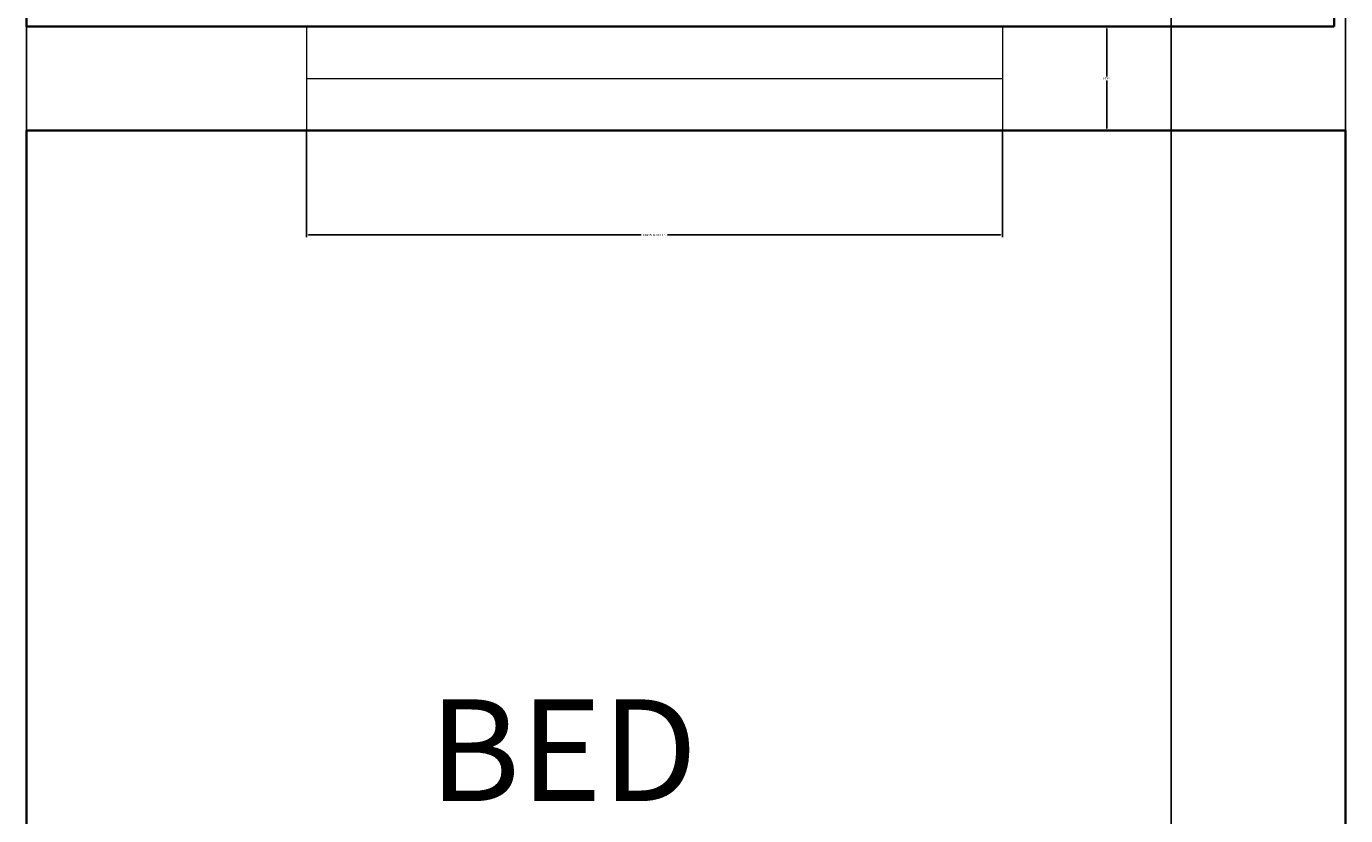
# Model space of a CAD drawing. Units: feet. Extents: x 100807 to 101423, y 154875 to 156331.
# Tile 5 of 8: x 101058 to 101172, y 156097 to 156166. Entities that reach past the tile are written whole.
import ezdxf

# ---------------------------------------------------------------- set-up
doc = ezdxf.new("R2010")
doc.units = ezdxf.units.FT
for name, color, linetype, lineweight in [('A-ANNO-DIMS', 2, 'Continuous', 18), ('A-AREA-IDEN', 7, 'Continuous', 25), ('A-GLAZ', 4, 'Continuous', 18), ('A-WALL', 7, 'Continuous', 35)]:
    doc.layers.add(name, color=color, linetype=linetype, lineweight=lineweight)
doc.styles.get("Standard").update_dxf_attribs({"font": 'arial.ttf'})
doc.dimstyles.get("Standard").update_dxf_attribs({"dimtxt": 0.18, "dimasz": 0.18, "dimexe": 0.18, "dimexo": 0.0625, "dimgap": 0.09, "dimtad": 0, "dimtih": 1, "dimtoh": 1, "dimdec": 4, "dimzin": 0, "dimdsep": 46, "dimtxsty": 'Standard', "dimcen": 0.09, "dimadec": 0, "dimazin": 0, "dimtfac": 1, "dimtdec": 4, "dimtofl": 0, "dimtmove": 0, "dimatfit": 3, "dimfxl": 1, "dimtolj": 1, "dimtzin": 0, "dimarcsym": 0})

# ---------------------------------------------------------------- blocks, each defined once
blk = doc.blocks.new('WIN-BED-END')
for p, q in [((0, 9), (0, 0)), ((60.14, 9), (60.14, 0)), ((0, 4.5), (60.14, 4.5))]:
    blk.add_line(p, q)
blk = doc.blocks.new('*D28')
at = {"layer": 'A-ANNO-DIMS', "color": 0, "lineweight": -2, "transparency": 16777216}
for p, q in [((101082.36, 156156.52), (101082.36, 156147.38)), ((101142.5, 156156.52), (101142.5, 156147.38)), ((101082.54, 156147.56), (101111.29, 156147.56)), ((101142.32, 156147.56), (101113.57, 156147.56))]:
    blk.add_line(p, q, dxfattribs=at)
at = {"layer": 'A-ANNO-DIMS', "color": 0, "transparency": 16777216}
for points in [[(101082.54, 156147.59), (101082.54, 156147.53), (101082.36, 156147.56)], [(101142.32, 156147.59), (101142.32, 156147.53), (101142.5, 156147.56)]]:
    blk.add_solid(points, dxfattribs=at)
at = {"layer": 'Defpoints', "color": 0, "transparency": 16777216}
for p in [(101082.36, 156156.58), (101142.5, 156156.58), (101142.5, 156147.56)]:
    blk.add_point(p, dxfattribs=at)
at = {"layer": 'A-ANNO-DIMS', "color": 0, "transparency": 16777216, "insert": (101112.43, 156147.56), "char_height": 0.18, "attachment_point": 5}
blk.add_mtext('\\A1;END WIN. 60 TYP.', dxfattribs=at)
blk = doc.blocks.new('*D29')
at = {"layer": 'A-ANNO-DIMS', "color": 0, "lineweight": -2, "transparency": 16777216}
for p, q in [((101142.56, 156165.58), (101151.7, 156165.58)), ((101151.52, 156165.4), (101151.52, 156161.26)), ((101151.52, 156156.76), (101151.52, 156160.9)), ((101142.56, 156156.58), (101151.7, 156156.58))]:
    blk.add_line(p, q, dxfattribs=at)
at = {"layer": 'A-ANNO-DIMS', "color": 0, "transparency": 16777216}
for points in [[(101151.49, 156165.4), (101151.55, 156165.4), (101151.52, 156165.58)], [(101151.49, 156156.76), (101151.55, 156156.76), (101151.52, 156156.58)]]:
    blk.add_solid(points, dxfattribs=at)
at = {"layer": 'Defpoints', "color": 0, "transparency": 16777216}
for p in [(101142.5, 156165.58), (101151.52, 156165.58), (101142.5, 156156.58)]:
    blk.add_point(p, dxfattribs=at)
at = {"layer": 'A-ANNO-DIMS', "color": 0, "transparency": 16777216, "insert": (101151.52, 156161.08), "char_height": 0.18, "attachment_point": 5}
blk.add_mtext('\\A1;9 TYP.', dxfattribs=at)
blk = doc.blocks.new('*D36')
at = {"layer": 'A-ANNO-DIMS', "color": 0, "lineweight": -2, "transparency": 16777216}
for p, q in [((101058.16, 155866.64), (101058.16, 156302.91)), ((101058.34, 156302.73), (101114.88, 156302.73)), ((101171.98, 156302.73), (101115.44, 156302.73)), ((101172.16, 155866.64), (101172.16, 156302.91))]:
    blk.add_line(p, q, dxfattribs=at)
at = {"layer": 'A-ANNO-DIMS', "color": 0, "transparency": 16777216}
for points in [[(101058.34, 156302.76), (101058.34, 156302.7), (101058.16, 156302.73)], [(101171.98, 156302.76), (101171.98, 156302.7), (101172.16, 156302.73)]]:
    blk.add_solid(points, dxfattribs=at)
at = {"layer": 'Defpoints', "color": 0, "transparency": 16777216}
for p in [(101172.16, 156302.73), (101058.16, 155866.58), (101172.16, 155866.58)]:
    blk.add_point(p, dxfattribs=at)
at = {"layer": 'A-ANNO-DIMS', "color": 0, "transparency": 16777216, "insert": (101115.16, 156302.73), "char_height": 0.18, "attachment_point": 5}
blk.add_mtext('\\A1;114', dxfattribs=at)
blk = doc.blocks.new('*D49')
at = {"layer": 'A-ANNO-DIMS', "color": 0, "lineweight": -2, "transparency": 16777216}
for p, q in [((101157.08, 155866.64), (101157.08, 156302.91)), ((101157.26, 156302.73), (101164.16, 156302.73)), ((101171.98, 156302.73), (101165.07, 156302.73)), ((101172.16, 155866.64), (101172.16, 156302.91))]:
    blk.add_line(p, q, dxfattribs=at)
at = {"layer": 'A-ANNO-DIMS', "color": 0, "transparency": 16777216}
for points in [[(101157.26, 156302.76), (101157.26, 156302.7), (101157.08, 156302.73)], [(101171.98, 156302.76), (101171.98, 156302.7), (101172.16, 156302.73)]]:
    blk.add_solid(points, dxfattribs=at)
at = {"layer": 'Defpoints', "color": 0, "transparency": 16777216}
for p in [(101172.16, 156302.73), (101157.08, 155866.58), (101172.16, 155866.58)]:
    blk.add_point(p, dxfattribs=at)
at = {"layer": 'A-ANNO-DIMS', "color": 0, "transparency": 16777216, "insert": (101164.62, 156302.73), "char_height": 0.18, "attachment_point": 5}
blk.add_mtext('\\A1;15.075', dxfattribs=at)

msp = doc.modelspace()

# ---------------------------------------------------------------- linework, layer by layer
at = {"layer": 'A-WALL'}
for p, q in [((101058.1564, 156234.5777), (101058.1564, 156165.5789)), ((101171.1564, 156234.5777), (101171.1564, 156165.5789)), ((101058.1564, 156165.5789), (101171.1564, 156165.5789)), ((101058.1564, 156156.5789), (101172.1564, 156156.5789)), ((101058.1564, 156156.5789), (101058.1564, 156068.7713)), ((101172.1564, 156156.5789), (101172.1564, 156032.5789))]:
    msp.add_line(p, q, dxfattribs=at)

# ---------------------------------------------------------------- block references
at = {"layer": 'A-GLAZ'}
msp.add_blockref('WIN-BED-END', (101082.3615, 156156.5789), dxfattribs=at)

# ---------------------------------------------------------------- texts
at = {"layer": 'A-AREA-IDEN'}
msp.add_text('BED', height=8.78822, dxfattribs=at).set_placement((101092.9589, 156098.6461))

# ---------------------------------------------------------------- dimensions: what is measured, and where the dimension line sits
at = {"layer": 'A-ANNO-DIMS'}
for p1, override, picture, middle in [((101058.1564, 155866.5789), {"dimdec": 0, "dimlfac": 1, "dimrnd": 0, "dimzin": 0, "dimdsep": 46, "dimlunit": 2}, '*D36', (101115.1564, 156302.7277)), ((101157.0816, 155866.5789), {"dimdec": 3, "dimlfac": 1, "dimrnd": 0, "dimzin": 0, "dimdsep": 46, "dimlunit": 2}, '*D49', (101164.619, 156302.7277))]:
    dim = msp.add_linear_dim(base=(101172.1564, 156302.7277), p1=p1, p2=(101172.1564, 155866.5789), dimstyle='Standard', override=override, dxfattribs=at)
    dim.commit()
    dim.dimension.update_dxf_attribs({"geometry": picture, "text_midpoint": middle})
dim = msp.add_linear_dim(base=(101151.5214, 156165.5789), p1=(101142.5006, 156156.5789), p2=(101142.5006, 156165.5789), angle=90, text='<> TYP.', dimstyle='Standard', override={"dimdec": 0, "dimlfac": 1, "dimrnd": 0, "dimzin": 0, "dimdsep": 46, "dimlunit": 2}, dxfattribs=at)
dim.commit()
dim.dimension.update_dxf_attribs({"geometry": '*D29', "text_midpoint": (101151.5214, 156161.0789)})
dim = msp.add_linear_dim(base=(101142.5006, 156147.5581), p1=(101082.3615, 156156.5789), p2=(101142.5006, 156156.5789), text='END WIN. <> TYP.', dimstyle='Standard', override={"dimdec": 0, "dimlfac": 1, "dimrnd": 0, "dimzin": 0, "dimdsep": 46, "dimlunit": 2}, dxfattribs=at)
dim.commit()
dim.dimension.update_dxf_attribs({"geometry": '*D28', "text_midpoint": (101112.431, 156147.5581)})

doc.saveas('drawing.dxf')
